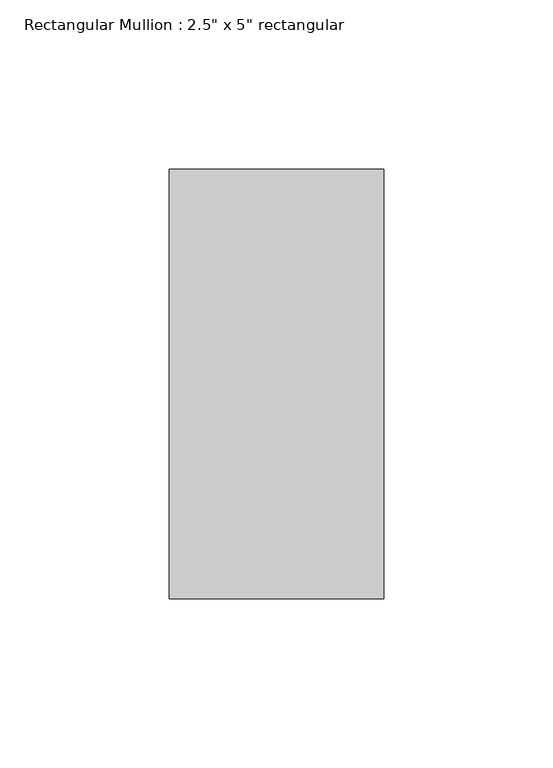
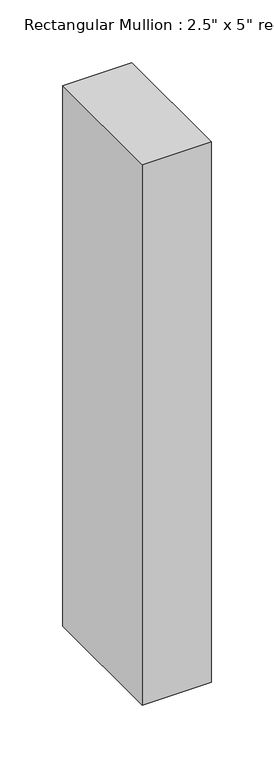
"""IFC4 building model written with IfcOpenShell, lengths in millimetres: member geometry."""

from ifc_helpers import new_model, si_unit, frame, origin, place, context, project, spatial, polyline, outline, extrude, source, transform, mapped, element, save


def member_b9da2caa(model_context):
    return source(origin(), model_context, "Body", "SweptSolid", [
        extrude(outline(polyline([(0.0, 63.5), (0.0, -63.5), (-63.5, -63.5), (-63.5, 63.5), (0.0, 63.5)])), frame((0.0, 0.0, -526.4018983), z_axis=(0.0, 0.0, 1.0), x_axis=(1.0, 0.0, 0.0)), (0.0, 0.0, 1.0), 526.4018983),
    ])


if __name__ == "__main__":
    model = new_model("IFC4")
    model_context = context("Model", 3, world=origin())
    ifc_project = project(units=[si_unit("LENGTHUNIT", "METRE", prefix="MILLI")], contexts=[model_context])
    site = spatial("IfcSite", under=ifc_project)
    building = spatial("IfcBuilding", under=site)
    placement = place(None, origin())
    member_shape = member_b9da2caa(model_context)
    element("IfcMember", 1, ObjectType="Rectangular Mullion : 2.5\" x 5\" rectangular", at=placement, inside=building, context=model_context, shape_type="MappedRepresentation", body=[
        mapped(member_shape, transform((0.0, 0.0, 0.0), x_axis=(1.0, 0.0, 0.0), y_axis=(0.0, 1.0, 0.0), z_axis=(0.0, 0.0, 1.0))),
    ])
    save(model, "model.ifc")

# Revit data of these elements
# Type "Rectangular Mullion : 2.5\" x 5\" rectangular"
#   built-in parameter 1007304 = 0.416667 (stored number, unit not read)
#   built-in parameter 1007301 = 0.104167 (stored number, unit not read)
#   built-in parameter 1007300 = 0.104167 (stored number, unit not read)
# Element 1 (IfcMember, "Rectangular Mullion : 2.5\" x 5\" rectangular")
#   Materials on its faces: "Aluminum"
# Materials
#   "Aluminum": class "Metal", colour RGB 247 247 247, transparency 0, Description = "Aluminum 6061", Cost = 0
